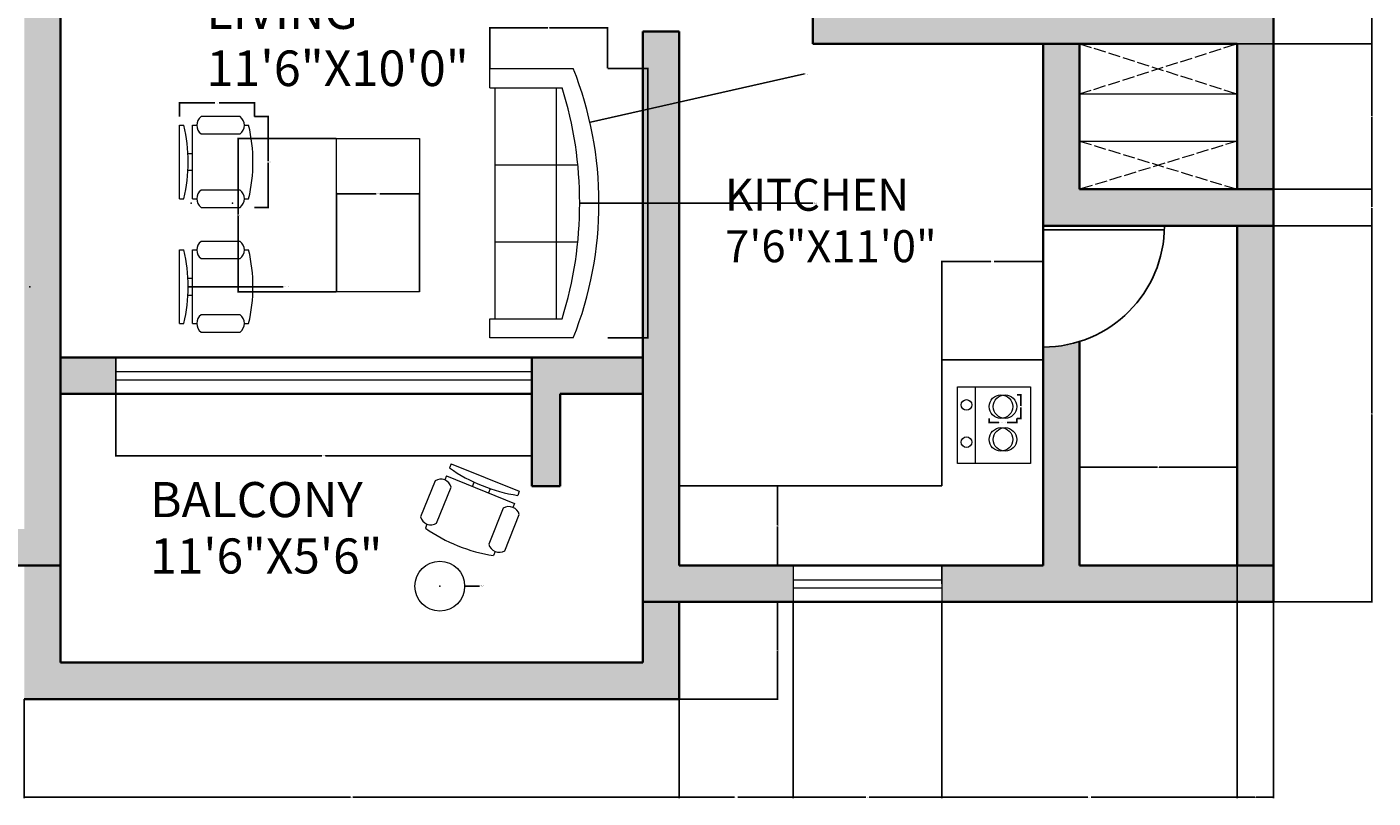
# Model space of a CAD drawing. Units: inches. Extents: x 582 to 1090, y 270 to 781.
# Tile 2 of 5: x 757 to 1090, y 270 to 461. Entities that reach past the tile are written whole.
import ezdxf

# ---------------------------------------------------------------- set-up
doc = ezdxf.new("R2010")
doc.units = ezdxf.units.IN
doc.header["$MEASUREMENT"] = 0
doc.linetypes.add('ACAD_ISO02W100', pattern=[15, 12, -3])
for name, color, linetype, lineweight in [('A-ANNO-DIMS', 2, 'Continuous', 18), ('A-AREA-IDEN', 7, 'Continuous', 25), ('A-DOOR', 3, 'Continuous', 25), ('A-EQPM', 8, 'Continuous', 18), ('A-FLOR-CASE', 32, 'Continuous', 25), ('A-FLOR-OPEN', 7, 'Continuous', 18), ('A-FLOR-OPEN-IDEN', 8, 'ACAD_ISO02W100', 13), ('A-FURN', 8, 'Continuous', 18), ('A-GLAZ', 4, 'Continuous', 18), ('A-WALL', 7, 'Continuous', 35)]:
    doc.layers.add(name, color=color, linetype=linetype, lineweight=lineweight)
doc.layers.add('A-WALL-PATT', color=9, linetype='Continuous', lineweight=13, true_color=0xc7c8ca)
doc.styles.get("Standard").update_dxf_attribs({"font": 'arial.ttf'})
doc.dimstyles.get("Standard").update_dxf_attribs({"dimtxt": 0.18, "dimasz": 0.18, "dimexe": 0.18, "dimexo": 0.0625, "dimgap": 0.09, "dimtad": 0, "dimtih": 1, "dimtoh": 1, "dimdec": 0, "dimzin": 0, "dimdsep": 46, "dimlunit": 3, "dimtxsty": 'Standard', "dimcen": 0.09, "dimadec": 0, "dimazin": 0, "dimtfac": 1, "dimtdec": 0, "dimtofl": 0, "dimtmove": 0, "dimatfit": 3, "dimfxl": 1, "dimtolj": 1, "dimtzin": 0, "dimarcsym": 0})

# ---------------------------------------------------------------- blocks, each defined once
blk = doc.blocks.new('Sofa - Roundback 7 ft.')
for p, q in [((-12.00002, -32.4421), (-12.00003, -6.5971)), ((11.99997, -32.4421), (11.99998, -6.5971)), ((-36.000027, -34), (-36.000027, -11.4696)), ((35.99998, -34), (35.99998, -11.4696)), ((-35.999844, -13.3819), (35.9998, -13.3819)), ((-36.000027, -32.4421), (35.99998, -32.4421))]:
    blk.add_line(p, q)
for points in [[(-36.000027, -34), (-42.000027, -34), (-42.000027, -8)], [(41.99998, -8), (41.99998, -34), (35.99998, -34)]]:
    blk.add_lwpolyline(points)
for centre, radius, start, end in [((0, -114.25), 114.25, 68.43141, 111.5686), ((-0.00001, -127.1968), 121.1968, 72.72033, 107.2797)]:
    blk.add_arc(centre, radius, start, end)
blk = doc.blocks.new('Chair - Desk')
for p, q in [((-8.5, 0), (-8.5, -1)), ((-8.5, 0), (8.5, 0)), ((8.5, 0), (8.5, -1)), ((-8.5, -3), (-8.5, -4)), ((-8.5, -3), (8.5, -3)), ((-2, -3), (-2, -1.9355)), ((2, -1.9576), (2, -3)), ((8.5, -3), (8.5, -4)), ((-10.5, -5), (-10.5, -14)), ((-6.5, -14), (-6.5, -5)), ((6.5, -5), (6.5, -14)), ((10.5, -14), (10.5, -5)), ((-8.5, -15), (-8.5, -16)), ((8.5, -15), (8.5, -16))]:
    blk.add_line(p, q)
for centre, radius, start, end in [((0, 34.625), 36.625, 256.5803, 283.4197), ((-8.5, -6.5), 2.5, 36.8699, 143.1301), ((8.5, -6.5), 2.5, 36.8699, 143.1301), ((-8.5, -12.5), 2.5, 216.8699, 323.1301), ((8.5, -12.5), 2.5, 216.8699, 323.1301), ((0, 19.625), 36.625, 256.5803, 283.4197)]:
    blk.add_arc(centre, radius, start, end)
blk = doc.blocks.new('DOOR-SINGLE-30IN')
for p, q in [((29, 0), (29, 30)), ((30, 0), (30, 30))]:
    blk.add_line(p, q)
blk.add_arc((30, 0), 30, 90, 180)
blk = doc.blocks.new('COOKTOP-BURNER')
for centre in [(2.91, 2.91), (3.92, 2.91)]:
    blk.add_circle(centre, 2.91)
blk = doc.blocks.new('*D22')
at = {"layer": 'A-ANNO-DIMS', "color": 0, "lineweight": -2, "transparency": 16777216}
for p, q in [((901.12, 450.33), (911.24, 450.33)), ((911.06, 450.15), (911.06, 417.2)), ((911.06, 383.89), (911.06, 416.84)), ((901.12, 383.71), (911.24, 383.71))]:
    blk.add_line(p, q, dxfattribs=at)
at = {"layer": 'A-ANNO-DIMS', "color": 0, "transparency": 16777216}
for points in [[(911.03, 450.15), (911.09, 450.15), (911.06, 450.33)], [(911.03, 383.89), (911.09, 383.89), (911.06, 383.71)]]:
    blk.add_solid(points, dxfattribs=at)
at = {"layer": 'Defpoints', "color": 0, "transparency": 16777216}
for p in [(901.06, 450.33), (901.06, 383.71), (911.06, 383.71)]:
    blk.add_point(p, dxfattribs=at)
at = {"layer": 'A-ANNO-DIMS', "color": 0, "transparency": 16777216, "insert": (911.06, 417.02), "char_height": 0.18, "attachment_point": 5}
blk.add_mtext('\\A1;SOFA 67', dxfattribs=at)
blk = doc.blocks.new('*D23')
at = {"layer": 'A-ANNO-DIMS', "color": 0, "lineweight": -2, "transparency": 16777216}
for p, q in [((871.98, 450.39), (871.98, 460.51)), ((872.16, 460.33), (886.3, 460.33)), ((900.88, 460.33), (886.74, 460.33)), ((901.06, 450.39), (901.06, 460.51))]:
    blk.add_line(p, q, dxfattribs=at)
at = {"layer": 'A-ANNO-DIMS', "color": 0, "transparency": 16777216}
for points in [[(872.16, 460.36), (872.16, 460.3), (871.98, 460.33)], [(900.88, 460.36), (900.88, 460.3), (901.06, 460.33)]]:
    blk.add_solid(points, dxfattribs=at)
at = {"layer": 'Defpoints', "color": 0, "transparency": 16777216}
for p in [(901.06, 460.33), (871.98, 450.33), (901.06, 450.33)]:
    blk.add_point(p, dxfattribs=at)
at = {"layer": 'A-ANNO-DIMS', "color": 0, "transparency": 16777216, "insert": (886.52, 460.33), "char_height": 0.18, "attachment_point": 5}
blk.add_mtext('\\A1;29', dxfattribs=at)
blk = doc.blocks.new('*D24')
at = {"layer": 'A-ANNO-DIMS', "color": 0, "lineweight": -2, "transparency": 16777216}
for p, q in [((813.79, 438.43), (817.28, 438.43)), ((817.1, 438.25), (817.1, 427.39)), ((817.1, 416.17), (817.1, 427.02)), ((813.79, 415.99), (817.28, 415.99))]:
    blk.add_line(p, q, dxfattribs=at)
at = {"layer": 'A-ANNO-DIMS', "color": 0, "transparency": 16777216}
for points in [[(817.07, 438.25), (817.13, 438.25), (817.1, 438.43)], [(817.07, 416.17), (817.13, 416.17), (817.1, 415.99)]]:
    blk.add_solid(points, dxfattribs=at)
at = {"layer": 'Defpoints', "color": 0, "transparency": 16777216}
for p in [(813.73, 438.43), (817.1, 438.43), (813.73, 415.99)]:
    blk.add_point(p, dxfattribs=at)
at = {"layer": 'A-ANNO-DIMS', "color": 0, "transparency": 16777216, "insert": (817.1, 427.21), "char_height": 0.18, "attachment_point": 5}
blk.add_mtext('\\A1;CHAIR 22 TYP.', dxfattribs=at)
blk = doc.blocks.new('*D25')
at = {"layer": 'A-ANNO-DIMS', "color": 0, "lineweight": -2, "transparency": 16777216}
for p, q in [((795.21, 438.49), (795.21, 441.97)), ((795.39, 441.79), (803.95, 441.79)), ((813.55, 441.79), (804.99, 441.79)), ((813.73, 438.49), (813.73, 441.97))]:
    blk.add_line(p, q, dxfattribs=at)
at = {"layer": 'A-ANNO-DIMS', "color": 0, "transparency": 16777216}
for points in [[(795.39, 441.82), (795.39, 441.76), (795.21, 441.79)], [(813.55, 441.82), (813.55, 441.76), (813.73, 441.79)]]:
    blk.add_solid(points, dxfattribs=at)
at = {"layer": 'Defpoints', "color": 0, "transparency": 16777216}
for p in [(795.21, 441.79), (795.21, 438.43), (813.73, 438.43)]:
    blk.add_point(p, dxfattribs=at)
at = {"layer": 'A-ANNO-DIMS', "color": 0, "transparency": 16777216, "insert": (804.47, 441.79), "char_height": 0.18, "attachment_point": 5}
blk.add_mtext('\\A1;19 TYP.', dxfattribs=at)
blk = doc.blocks.new('*D32')
at = {"layer": 'A-ANNO-DIMS', "color": 0, "lineweight": -2, "transparency": 16777216}
for p, q in [((995.45, 363.75), (995.45, 362.61)), ((1002.28, 363.75), (1002.28, 362.61)), ((995.63, 362.79), (997.85, 362.79)), ((1002.1, 362.79), (999.89, 362.79))]:
    blk.add_line(p, q, dxfattribs=at)
at = {"layer": 'A-ANNO-DIMS', "color": 0, "transparency": 16777216}
for points in [[(995.63, 362.82), (995.63, 362.76), (995.45, 362.79)], [(1002.1, 362.82), (1002.1, 362.76), (1002.28, 362.79)]]:
    blk.add_solid(points, dxfattribs=at)
at = {"layer": 'Defpoints', "color": 0, "transparency": 16777216}
for p in [(995.45, 363.81), (1002.28, 363.81), (1002.28, 362.79)]:
    blk.add_point(p, dxfattribs=at)
at = {"layer": 'A-ANNO-DIMS', "color": 0, "transparency": 16777216, "insert": (998.87, 362.79), "char_height": 0.18, "attachment_point": 5}
blk.add_mtext('\\A1;BURNER 7 TYP.', dxfattribs=at)
blk = doc.blocks.new('*D33')
at = {"layer": 'A-ANNO-DIMS', "color": 0, "lineweight": -2, "transparency": 16777216}
for p, q in [((1002.35, 369.64), (1003.49, 369.64)), ((1003.31, 369.46), (1003.31, 366.91)), ((1003.31, 363.99), (1003.31, 366.54)), ((1002.35, 363.81), (1003.49, 363.81))]:
    blk.add_line(p, q, dxfattribs=at)
at = {"layer": 'A-ANNO-DIMS', "color": 0, "transparency": 16777216}
for points in [[(1003.28, 369.46), (1003.34, 369.46), (1003.31, 369.64)], [(1003.28, 363.99), (1003.34, 363.99), (1003.31, 363.81)]]:
    blk.add_solid(points, dxfattribs=at)
at = {"layer": 'Defpoints', "color": 0, "transparency": 16777216}
for p in [(1002.28, 369.64), (1003.31, 369.64), (1002.28, 363.81)]:
    blk.add_point(p, dxfattribs=at)
at = {"layer": 'A-ANNO-DIMS', "color": 0, "transparency": 16777216, "insert": (1003.31, 366.72), "char_height": 0.18, "attachment_point": 5}
blk.add_mtext('\\A1;6 TYP.', dxfattribs=at)
blk = doc.blocks.new('*D38')
at = {"layer": 'A-ANNO-DIMS', "color": 0, "lineweight": -2, "transparency": 16777216}
for p, q in [((918.87, 318.45), (943.28, 318.45)), ((943.1, 318.27), (943.1, 306.62)), ((943.1, 294.62), (943.1, 306.26)), ((918.87, 294.44), (943.28, 294.44))]:
    blk.add_line(p, q, dxfattribs=at)
at = {"layer": 'A-ANNO-DIMS', "color": 0, "transparency": 16777216}
for points in [[(943.07, 318.27), (943.13, 318.27), (943.1, 318.45)], [(943.07, 294.62), (943.13, 294.62), (943.1, 294.44)]]:
    blk.add_solid(points, dxfattribs=at)
at = {"layer": 'Defpoints', "color": 0, "transparency": 16777216}
for p in [(918.8, 318.45), (918.8, 294.44), (943.1, 294.44)]:
    blk.add_point(p, dxfattribs=at)
at = {"layer": 'A-ANNO-DIMS', "color": 0, "transparency": 16777216, "insert": (943.1, 306.44), "char_height": 0.18, "attachment_point": 5}
blk.add_mtext('\\A1;24.01', dxfattribs=at)
blk = doc.blocks.new('*D39')
at = {"layer": 'A-ANNO-DIMS', "color": 0, "lineweight": -2, "transparency": 16777216}
for p, q in [((756.8, 294.37), (756.8, 269.96)), ((918.8, 294.37), (918.8, 269.96)), ((756.98, 270.14), (837.53, 270.14)), ((918.62, 270.14), (838.08, 270.14))]:
    blk.add_line(p, q, dxfattribs=at)
at = {"layer": 'A-ANNO-DIMS', "color": 0, "transparency": 16777216}
for points in [[(756.98, 270.17), (756.98, 270.11), (756.8, 270.14)], [(918.62, 270.17), (918.62, 270.11), (918.8, 270.14)]]:
    blk.add_solid(points, dxfattribs=at)
at = {"layer": 'Defpoints', "color": 0, "transparency": 16777216}
for p in [(756.8, 294.44), (918.8, 294.44), (918.8, 270.14)]:
    blk.add_point(p, dxfattribs=at)
at = {"layer": 'A-ANNO-DIMS', "color": 0, "transparency": 16777216, "insert": (837.8, 270.14), "char_height": 0.18, "attachment_point": 5}
blk.add_mtext('\\A1;162', dxfattribs=at)
blk = doc.blocks.new('*D43')
at = {"layer": 'A-ANNO-DIMS', "color": 0, "lineweight": -2, "transparency": 16777216}
for p, q in [((918.8, 318.38), (918.8, 269.96)), ((946.96, 318.38), (946.96, 269.96)), ((918.98, 270.14), (932.49, 270.14)), ((946.78, 270.14), (933.28, 270.14))]:
    blk.add_line(p, q, dxfattribs=at)
at = {"layer": 'A-ANNO-DIMS', "color": 0, "transparency": 16777216}
for points in [[(918.98, 270.17), (918.98, 270.11), (918.8, 270.14)], [(946.78, 270.17), (946.78, 270.11), (946.96, 270.14)]]:
    blk.add_solid(points, dxfattribs=at)
at = {"layer": 'Defpoints', "color": 0, "transparency": 16777216}
for p in [(918.8, 318.45), (946.96, 318.45), (946.96, 270.14)]:
    blk.add_point(p, dxfattribs=at)
at = {"layer": 'A-ANNO-DIMS', "color": 0, "transparency": 16777216, "insert": (932.88, 270.14), "char_height": 0.18, "attachment_point": 5}
blk.add_mtext('\\A1;28.16', dxfattribs=at)
blk = doc.blocks.new('*D44')
at = {"layer": 'A-ANNO-DIMS', "color": 0, "lineweight": -2, "transparency": 16777216}
for p, q in [((946.96, 318.38), (946.96, 269.96)), ((983.73, 318.38), (983.73, 269.96)), ((947.14, 270.14), (964.95, 270.14)), ((983.55, 270.14), (965.74, 270.14))]:
    blk.add_line(p, q, dxfattribs=at)
at = {"layer": 'A-ANNO-DIMS', "color": 0, "transparency": 16777216}
for points in [[(947.14, 270.17), (947.14, 270.11), (946.96, 270.14)], [(983.55, 270.17), (983.55, 270.11), (983.73, 270.14)]]:
    blk.add_solid(points, dxfattribs=at)
at = {"layer": 'Defpoints', "color": 0, "transparency": 16777216}
for p in [(946.96, 318.45), (983.73, 318.45), (983.73, 270.14)]:
    blk.add_point(p, dxfattribs=at)
at = {"layer": 'A-ANNO-DIMS', "color": 0, "transparency": 16777216, "insert": (965.35, 270.14), "char_height": 0.18, "attachment_point": 5}
blk.add_mtext('\\A1;36.77', dxfattribs=at)
blk = doc.blocks.new('*D45')
at = {"layer": 'A-ANNO-DIMS', "color": 0, "lineweight": -2, "transparency": 16777216}
for p, q in [((1056.8, 327.38), (1056.8, 269.96)), ((983.73, 318.38), (983.73, 269.96)), ((983.91, 270.14), (1019.88, 270.14)), ((1056.62, 270.14), (1020.66, 270.14))]:
    blk.add_line(p, q, dxfattribs=at)
at = {"layer": 'A-ANNO-DIMS', "color": 0, "transparency": 16777216}
for points in [[(983.91, 270.17), (983.91, 270.11), (983.73, 270.14)], [(1056.62, 270.17), (1056.62, 270.11), (1056.8, 270.14)]]:
    blk.add_solid(points, dxfattribs=at)
at = {"layer": 'Defpoints', "color": 0, "transparency": 16777216}
for p in [(1056.8, 327.45), (983.73, 318.45), (1056.8, 270.14)]:
    blk.add_point(p, dxfattribs=at)
at = {"layer": 'A-ANNO-DIMS', "color": 0, "transparency": 16777216, "insert": (1020.27, 270.14), "char_height": 0.18, "attachment_point": 5}
blk.add_mtext('\\A1;73.07', dxfattribs=at)
blk = doc.blocks.new('*D46')
at = {"layer": 'A-ANNO-DIMS', "color": 0, "lineweight": -2, "transparency": 16777216}
for p, q in [((1056.8, 327.38), (1056.8, 269.96)), ((1065.8, 318.38), (1065.8, 269.96)), ((1056.98, 270.14), (1061.16, 270.14)), ((1065.62, 270.14), (1061.45, 270.14))]:
    blk.add_line(p, q, dxfattribs=at)
at = {"layer": 'A-ANNO-DIMS', "color": 0, "transparency": 16777216}
for points in [[(1056.98, 270.17), (1056.98, 270.11), (1056.8, 270.14)], [(1065.62, 270.17), (1065.62, 270.11), (1065.8, 270.14)]]:
    blk.add_solid(points, dxfattribs=at)
at = {"layer": 'Defpoints', "color": 0, "transparency": 16777216}
for p in [(1056.8, 327.45), (1065.8, 318.45), (1065.8, 270.14)]:
    blk.add_point(p, dxfattribs=at)
at = {"layer": 'A-ANNO-DIMS', "color": 0, "transparency": 16777216, "insert": (1061.3, 270.14), "char_height": 0.18, "attachment_point": 5}
blk.add_mtext('\\A1;9', dxfattribs=at)
blk = doc.blocks.new('*D47')
at = {"layer": 'A-ANNO-DIMS', "color": 0, "lineweight": -2, "transparency": 16777216}
for p, q in [((779.42, 378.81), (779.42, 354.39)), ((882.35, 378.81), (882.35, 354.39)), ((779.6, 354.57), (830.43, 354.57)), ((882.17, 354.57), (831.34, 354.57))]:
    blk.add_line(p, q, dxfattribs=at)
at = {"layer": 'A-ANNO-DIMS', "color": 0, "transparency": 16777216}
for points in [[(779.6, 354.6), (779.6, 354.54), (779.42, 354.57)], [(882.17, 354.6), (882.17, 354.54), (882.35, 354.57)]]:
    blk.add_solid(points, dxfattribs=at)
at = {"layer": 'Defpoints', "color": 0, "transparency": 16777216}
for p in [(779.42, 378.87), (882.35, 378.87), (779.42, 354.57)]:
    blk.add_point(p, dxfattribs=at)
at = {"layer": 'A-ANNO-DIMS', "color": 0, "transparency": 16777216, "insert": (830.89, 354.57), "char_height": 0.18, "attachment_point": 5}
blk.add_mtext('\\A1;102.93', dxfattribs=at)
blk = doc.blocks.new('*D58')
at = {"layer": 'A-ANNO-DIMS', "color": 0, "lineweight": -2, "transparency": 16777216}
for p, q in [((1065.87, 478.21), (1090.28, 478.21)), ((1090.1, 478.03), (1090.1, 467.51)), ((1090.1, 456.63), (1090.1, 467.15)), ((1056.87, 456.45), (1090.28, 456.45))]:
    blk.add_line(p, q, dxfattribs=at)
at = {"layer": 'A-ANNO-DIMS', "color": 0, "transparency": 16777216}
for points in [[(1090.07, 478.03), (1090.13, 478.03), (1090.1, 478.21)], [(1090.07, 456.63), (1090.13, 456.63), (1090.1, 456.45)]]:
    blk.add_solid(points, dxfattribs=at)
at = {"layer": 'Defpoints', "color": 0, "transparency": 16777216}
for p in [(1065.8, 478.21), (1090.1, 478.21), (1056.8, 456.45)]:
    blk.add_point(p, dxfattribs=at)
at = {"layer": 'A-ANNO-DIMS', "color": 0, "transparency": 16777216, "insert": (1090.1, 467.33), "char_height": 0.18, "attachment_point": 5}
blk.add_mtext('\\A1;21.77', dxfattribs=at)
blk = doc.blocks.new('*D59')
at = {"layer": 'A-ANNO-DIMS', "color": 0, "lineweight": -2, "transparency": 16777216}
for p, q in [((1056.87, 456.45), (1090.28, 456.45)), ((1090.1, 456.27), (1090.1, 438.63)), ((1090.1, 420.63), (1090.1, 438.26)), ((1056.87, 420.45), (1090.28, 420.45))]:
    blk.add_line(p, q, dxfattribs=at)
at = {"layer": 'A-ANNO-DIMS', "color": 0, "transparency": 16777216}
for points in [[(1090.07, 456.27), (1090.13, 456.27), (1090.1, 456.45)], [(1090.07, 420.63), (1090.13, 420.63), (1090.1, 420.45)]]:
    blk.add_solid(points, dxfattribs=at)
at = {"layer": 'Defpoints', "color": 0, "transparency": 16777216}
for p in [(1056.8, 456.45), (1090.1, 456.45), (1056.8, 420.45)]:
    blk.add_point(p, dxfattribs=at)
at = {"layer": 'A-ANNO-DIMS', "color": 0, "transparency": 16777216, "insert": (1090.1, 438.45), "char_height": 0.18, "attachment_point": 5}
blk.add_mtext('\\A1;36', dxfattribs=at)
blk = doc.blocks.new('*D60')
at = {"layer": 'A-ANNO-DIMS', "color": 0, "lineweight": -2, "transparency": 16777216}
for p, q in [((1056.87, 420.45), (1090.28, 420.45)), ((1090.1, 420.27), (1090.1, 416.13)), ((1090.1, 411.63), (1090.1, 415.76)), ((1065.87, 411.45), (1090.28, 411.45))]:
    blk.add_line(p, q, dxfattribs=at)
at = {"layer": 'A-ANNO-DIMS', "color": 0, "transparency": 16777216}
for points in [[(1090.07, 420.27), (1090.13, 420.27), (1090.1, 420.45)], [(1090.07, 411.63), (1090.13, 411.63), (1090.1, 411.45)]]:
    blk.add_solid(points, dxfattribs=at)
at = {"layer": 'Defpoints', "color": 0, "transparency": 16777216}
for p in [(1056.8, 420.45), (1090.1, 420.45), (1065.8, 411.45)]:
    blk.add_point(p, dxfattribs=at)
at = {"layer": 'A-ANNO-DIMS', "color": 0, "transparency": 16777216, "insert": (1090.1, 415.95), "char_height": 0.18, "attachment_point": 5}
blk.add_mtext('\\A1;9', dxfattribs=at)
blk = doc.blocks.new('*D61')
at = {"layer": 'A-ANNO-DIMS', "color": 0, "lineweight": -2, "transparency": 16777216}
for p, q in [((1065.87, 411.45), (1090.28, 411.45)), ((1090.1, 411.27), (1090.1, 365.13)), ((1090.1, 318.63), (1090.1, 364.76)), ((1065.87, 318.45), (1090.28, 318.45))]:
    blk.add_line(p, q, dxfattribs=at)
at = {"layer": 'A-ANNO-DIMS', "color": 0, "transparency": 16777216}
for points in [[(1090.07, 411.27), (1090.13, 411.27), (1090.1, 411.45)], [(1090.07, 318.63), (1090.13, 318.63), (1090.1, 318.45)]]:
    blk.add_solid(points, dxfattribs=at)
at = {"layer": 'Defpoints', "color": 0, "transparency": 16777216}
for p in [(1065.8, 411.45), (1090.1, 411.45), (1065.8, 318.45)]:
    blk.add_point(p, dxfattribs=at)
at = {"layer": 'A-ANNO-DIMS', "color": 0, "transparency": 16777216, "insert": (1090.1, 364.95), "char_height": 0.18, "attachment_point": 5}
blk.add_mtext('\\A1;93', dxfattribs=at)
blk = doc.blocks.new('*D62')
at = {"layer": 'A-ANNO-DIMS', "color": 0, "lineweight": -2, "transparency": 16777216}
for p, q in [((1017.8, 327.51), (1017.8, 351.93)), ((1017.98, 351.75), (1037.09, 351.75)), ((1056.62, 351.75), (1037.52, 351.75)), ((1056.8, 327.51), (1056.8, 351.93))]:
    blk.add_line(p, q, dxfattribs=at)
at = {"layer": 'A-ANNO-DIMS', "color": 0, "transparency": 16777216}
for points in [[(1017.98, 351.78), (1017.98, 351.72), (1017.8, 351.75)], [(1056.62, 351.78), (1056.62, 351.72), (1056.8, 351.75)]]:
    blk.add_solid(points, dxfattribs=at)
at = {"layer": 'Defpoints', "color": 0, "transparency": 16777216}
for p in [(1056.8, 351.75), (1017.8, 327.45), (1056.8, 327.45)]:
    blk.add_point(p, dxfattribs=at)
at = {"layer": 'A-ANNO-DIMS', "color": 0, "transparency": 16777216, "insert": (1037.3, 351.75), "char_height": 0.18, "attachment_point": 5}
blk.add_mtext('\\A1;39', dxfattribs=at)
blk = doc.blocks.new('*D63')
at = {"layer": 'A-ANNO-DIMS', "color": 0, "lineweight": -2, "transparency": 16777216}
for p, q in [((834.01, 395.13), (834.01, 419.55)), ((854.57, 395.13), (854.57, 419.55)), ((834.19, 419.37), (843.82, 419.37)), ((854.39, 419.37), (844.75, 419.37))]:
    blk.add_line(p, q, dxfattribs=at)
at = {"layer": 'A-ANNO-DIMS', "color": 0, "transparency": 16777216}
for points in [[(834.19, 419.4), (834.19, 419.34), (834.01, 419.37)], [(854.39, 419.4), (854.39, 419.34), (854.57, 419.37)]]:
    blk.add_solid(points, dxfattribs=at)
at = {"layer": 'Defpoints', "color": 0, "transparency": 16777216}
for p in [(854.57, 419.37), (834.01, 395.07), (854.57, 395.07)]:
    blk.add_point(p, dxfattribs=at)
at = {"layer": 'A-ANNO-DIMS', "color": 0, "transparency": 16777216, "insert": (844.29, 419.37), "char_height": 0.18, "attachment_point": 5}
blk.add_mtext('\\A1;20.563', dxfattribs=at)
blk = doc.blocks.new('*D64')
at = {"layer": 'A-ANNO-DIMS', "color": 0, "lineweight": -2, "transparency": 16777216}
for p, q in [((833.94, 433.04), (809.53, 433.04)), ((809.71, 432.86), (809.71, 414.24)), ((809.71, 395.25), (809.71, 413.87)), ((833.94, 395.07), (809.53, 395.07))]:
    blk.add_line(p, q, dxfattribs=at)
at = {"layer": 'A-ANNO-DIMS', "color": 0, "transparency": 16777216}
for points in [[(809.68, 432.86), (809.74, 432.86), (809.71, 433.04)], [(809.68, 395.25), (809.74, 395.25), (809.71, 395.07)]]:
    blk.add_solid(points, dxfattribs=at)
at = {"layer": 'Defpoints', "color": 0, "transparency": 16777216}
for p in [(809.71, 433.04), (834.01, 433.04), (834.01, 395.07)]:
    blk.add_point(p, dxfattribs=at)
at = {"layer": 'A-ANNO-DIMS', "color": 0, "transparency": 16777216, "insert": (809.71, 414.05), "char_height": 0.18, "attachment_point": 5}
blk.add_mtext('\\A1;37.98', dxfattribs=at)
blk = doc.blocks.new('*D65')
at = {"layer": 'A-ANNO-DIMS', "color": 0, "lineweight": -2, "transparency": 16777216}
for p, q in [((983.77, 378.34), (983.77, 402.76)), ((983.95, 402.58), (995.89, 402.58)), ((1008.62, 402.58), (996.68, 402.58)), ((1008.8, 378.34), (1008.8, 402.76))]:
    blk.add_line(p, q, dxfattribs=at)
at = {"layer": 'A-ANNO-DIMS', "color": 0, "transparency": 16777216}
for points in [[(983.95, 402.61), (983.95, 402.55), (983.77, 402.58)], [(1008.62, 402.61), (1008.62, 402.55), (1008.8, 402.58)]]:
    blk.add_solid(points, dxfattribs=at)
at = {"layer": 'Defpoints', "color": 0, "transparency": 16777216}
for p in [(1008.8, 402.58), (983.77, 378.28), (1008.8, 378.28)]:
    blk.add_point(p, dxfattribs=at)
at = {"layer": 'A-ANNO-DIMS', "color": 0, "transparency": 16777216, "insert": (996.29, 402.58), "char_height": 0.18, "attachment_point": 5}
blk.add_mtext('\\A1;25.03', dxfattribs=at)
blk = doc.blocks.new('*D66')
at = {"layer": 'A-ANNO-DIMS', "color": 0, "lineweight": -2, "transparency": 16777216}
for p, q in [((918.87, 347.11), (943.28, 347.11)), ((943.1, 346.93), (943.1, 337.46)), ((943.1, 327.63), (943.1, 337.1)), ((918.87, 327.45), (943.28, 327.45))]:
    blk.add_line(p, q, dxfattribs=at)
at = {"layer": 'A-ANNO-DIMS', "color": 0, "transparency": 16777216}
for points in [[(943.07, 346.93), (943.13, 346.93), (943.1, 347.11)], [(943.07, 327.63), (943.13, 327.63), (943.1, 327.45)]]:
    blk.add_solid(points, dxfattribs=at)
at = {"layer": 'Defpoints', "color": 0, "transparency": 16777216}
for p in [(918.8, 347.11), (918.8, 327.45), (943.1, 327.45)]:
    blk.add_point(p, dxfattribs=at)
at = {"layer": 'A-ANNO-DIMS', "color": 0, "transparency": 16777216, "insert": (943.1, 337.28), "char_height": 0.18, "attachment_point": 5}
blk.add_mtext('\\A1;19.668', dxfattribs=at)
blk = doc.blocks.new('*D67')
at = {"layer": 'A-ANNO-DIMS', "color": 0, "lineweight": -2, "transparency": 16777216}
for p, q in [((859.48, 322.35), (859.66, 322.35)), ((859.57, 322.26), (859.57, 322.44)), ((869.43, 322.35), (865.91, 322.35))]:
    blk.add_line(p, q, dxfattribs=at)
at = {"layer": 'A-ANNO-DIMS', "color": 0, "transparency": 16777216}
blk.add_solid([(865.91, 322.38), (865.91, 322.32), (865.73, 322.35)], dxfattribs=at)
at = {"layer": 'Defpoints', "color": 0, "transparency": 16777216}
for p in [(853.41, 322.34), (865.73, 322.35)]:
    blk.add_point(p, dxfattribs=at)
at = {"layer": 'A-ANNO-DIMS', "color": 0, "transparency": 16777216, "insert": (869.99, 322.35), "char_height": 0.18, "attachment_point": 5}
blk.add_mtext('\\A1;∅12.317', dxfattribs=at)
blk = doc.blocks.new('*D70')
at = {"layer": 'A-ANNO-DIMS', "color": 0, "lineweight": -2, "transparency": 16777216}
for p, q in [((797.97, 417.02), (798.15, 417.02)), ((798.06, 416.93), (798.06, 417.11)), ((951.86, 417.02), (894.37, 417.02))]:
    blk.add_line(p, q, dxfattribs=at)
at = {"layer": 'A-ANNO-DIMS', "color": 0, "transparency": 16777216}
blk.add_solid([(894.37, 417.05), (894.37, 416.99), (894.19, 417.02)], dxfattribs=at)
at = {"layer": 'Defpoints', "color": 0, "transparency": 16777216}
for p in [(798.06, 417.02), (894.19, 417.02)]:
    blk.add_point(p, dxfattribs=at)
at = {"layer": 'A-ANNO-DIMS', "color": 0, "transparency": 16777216, "insert": (952.34, 417.02), "char_height": 0.18, "attachment_point": 5}
blk.add_mtext('\\A1;R96.13', dxfattribs=at)
blk = doc.blocks.new('*D73')
at = {"layer": 'A-ANNO-DIMS', "color": 0, "lineweight": -2, "transparency": 16777216}
for p, q in [((949.75, 448.98), (896.89, 437.03)), ((808.24, 417.02), (808.42, 417.02)), ((808.33, 416.93), (808.33, 417.11))]:
    blk.add_line(p, q, dxfattribs=at)
at = {"layer": 'A-ANNO-DIMS', "color": 0, "transparency": 16777216}
blk.add_solid([(896.89, 437.06), (896.9, 437), (896.72, 436.99)], dxfattribs=at)
at = {"layer": 'Defpoints', "color": 0, "transparency": 16777216}
for p in [(896.72, 436.99), (808.33, 417.02)]:
    blk.add_point(p, dxfattribs=at)
at = {"layer": 'A-ANNO-DIMS', "color": 0, "transparency": 16777216, "insert": (950.23, 448.98), "char_height": 0.18, "attachment_point": 5}
blk.add_mtext('\\A1;R90.62', dxfattribs=at)
blk = doc.blocks.new('*D77')
at = {"layer": 'A-ANNO-DIMS', "color": 0, "lineweight": -2, "transparency": 16777216}
for p, q in [((758.12, 396.37), (758.3, 396.37)), ((758.21, 396.28), (758.21, 396.46)), ((820.83, 396.37), (797.53, 396.37))]:
    blk.add_line(p, q, dxfattribs=at)
at = {"layer": 'A-ANNO-DIMS', "color": 0, "transparency": 16777216}
blk.add_solid([(797.53, 396.4), (797.53, 396.34), (797.35, 396.37)], dxfattribs=at)
at = {"layer": 'Defpoints', "color": 0, "transparency": 16777216}
for p in [(758.21, 396.37), (797.35, 396.37)]:
    blk.add_point(p, dxfattribs=at)
at = {"layer": 'A-ANNO-DIMS', "color": 0, "transparency": 16777216, "insert": (821.57, 396.37), "char_height": 0.18, "attachment_point": 5}
blk.add_mtext('\\A1;6X R39.136', dxfattribs=at)

msp = doc.modelspace()

# ---------------------------------------------------------------- hatches: boundary and pattern name
at = {"layer": 'A-WALL-PATT'}
h = msp.add_hatch(color=256, dxfattribs=at)
h.dxf.hatch_style = 1
h.paths.add_polyline_path([(867.8047, 744.446), (765.8047, 744.446), (606.8047, 744.446), (606.8047, 711.9379), (615.8047, 711.9379), (615.8047, 735.446), (756.8047, 735.446), (756.8047, 585.446), (765.8047, 585.446), (765.8047, 735.446), (868.9478, 735.446, -0.06325422)])
h.paths.add_polyline_path([(1065.8047, 744.446), (912.8047, 744.446), (903.8047, 744.446), (903.8047, 708.446), (903.8047, 594.446), (903.8047, 564.6071), (912.8047, 564.6071), (912.8047, 600.6071), (912.8047, 735.446), (1056.8047, 735.446), (1056.8047, 720.2375), (1065.8047, 720.2375)])
h.paths.add_polyline_path([(1065.8047, 632.4383), (1056.8047, 632.4383), (1056.8047, 594.446), (1056.8047, 584.9343), (1065.8047, 584.9343), (1065.8047, 594.446)], flags=17)
h.paths.add_polyline_path([(1056.8047, 603.446), (951.8047, 603.446), (951.8047, 594.446), (1056.8047, 594.446)], flags=17)
h.paths.add_polyline_path([(1065.8047, 525.446), (1065.8047, 550.2593), (1056.8047, 550.2593), (1056.8047, 534.446), (960.8047, 534.446), (960.8047, 565.946, -0.07397332), (952.1262, 564.6071), (951.8047, 564.6071), (951.8047, 495.446, -0.07632083), (960.8047, 494.0641), (960.8047, 525.446), (1056.8047, 525.446), (1056.8047, 508.8565), (1065.8047, 508.8565)])
h.paths.add_polyline_path([(1065.8047, 478.2143), (1056.8047, 478.2143), (1056.8047, 465.446), (951.8047, 465.446), (951.8047, 456.446), (1056.8047, 456.446), (1056.8047, 420.446), (1065.8047, 420.446), (1065.8047, 456.446)])
h.paths.add_polyline_path([(1065.8047, 420.446), (1056.8047, 420.446), (1017.8047, 420.446), (1017.8047, 456.446), (1008.8047, 456.446), (1008.8047, 411.446), (1038.8047, 411.446), (1065.8047, 411.446)])
h.paths.add_polyline_path([(1065.8047, 411.446), (1056.8047, 411.446), (1056.8047, 327.446), (1065.8047, 327.446)])
h.paths.add_polyline_path([(1065.8047, 327.446), (1056.8047, 327.446), (1017.8047, 327.446), (1017.8047, 382.8278, -0.07632083), (1008.8047, 381.446), (1008.8047, 327.446), (983.7348, 327.446), (983.7348, 318.446), (1065.8047, 318.446)])
h.paths.add_polyline_path([(946.9624, 327.446), (918.8047, 327.446), (918.8047, 369.8742), (918.8047, 459.446), (909.8047, 459.446), (909.8047, 369.8742), (909.8047, 318.446), (946.9624, 318.446)])
h.paths.add_polyline_path([(918.8047, 318.446), (909.8047, 318.446), (909.8047, 303.4372), (765.8047, 303.4372), (765.8047, 327.446), (756.8047, 327.446), (756.8047, 294.4372), (918.8047, 294.4372)])
h.paths.add_polyline_path([(909.8047, 378.8742), (882.3477, 378.8742), (882.3477, 347.0959), (889.3299, 347.0959), (889.3299, 369.8742), (909.8047, 369.8742)])
h.paths.add_polyline_path([(779.4225, 378.8742), (765.8047, 378.8742), (765.8047, 369.8742), (779.4225, 369.8742)])
h.paths.add_polyline_path([(765.8047, 516.446), (756.8047, 516.446), (756.8047, 480.446), (756.8047, 336.446), (724.1731, 336.446), (724.1731, 327.446), (765.8047, 327.446), (765.8047, 369.8742), (765.8047, 378.8742)])
h.paths.add_polyline_path([(615.8047, 516.446), (606.8047, 516.446), (606.8047, 327.446), (637.062, 327.446), (637.062, 336.446), (615.8047, 336.446)])
h.paths.add_polyline_path([(615.8047, 631.6498), (606.8047, 631.6498), (606.8047, 585.446), (606.8047, 569.338), (615.8047, 569.338), (615.8047, 585.446), (615.8047, 594.446)])
h.paths.add_polyline_path([(721.9478, 594.446), (615.8047, 594.446), (615.8047, 585.446), (627.9505, 585.446, -0.03261849), (629.8936, 585.446), (710.8047, 585.446), (710.8047, 525.446), (675.3033, 525.446), (675.3033, 516.446), (719.8047, 516.446), (720.8047, 516.446), (720.8047, 525.446), (719.8047, 525.446), (719.8047, 585.446), (720.8047, 585.446, -0.06325422)])
h.paths.add_polyline_path([(646.6852, 525.446), (615.8047, 525.446), (615.8047, 516.446), (645.3033, 516.446, -0.07632083)])
h.paths.add_polyline_path([(615.8047, 525.446), (615.8047, 539.7667), (606.8047, 539.7667), (606.8047, 516.446), (615.8047, 516.446)])

# ---------------------------------------------------------------- linework, layer by layer
at = {"layer": 'A-DOOR'}
msp.add_line((1008.8047, 411.446), (1008.8047, 381.446), dxfattribs=at)
at = {"layer": 'A-EQPM'}
msp.add_line((991.9866, 371.6418), (991.9866, 352.7025), dxfattribs=at)
msp.add_lwpolyline([(987.6109, 371.6418), (1005.6608, 371.6418), (1005.6608, 352.7025), (987.6109, 352.7025)], close=True, dxfattribs=at)
for centre in [(989.8491, 367.1465), (989.8491, 357.9529)]:
    msp.add_circle(centre, 1.3124, dxfattribs=at)
at = {"layer": 'A-FLOR-CASE'}
for p, q in [((1008.8047, 378.277), (983.7733, 378.277)), ((983.7733, 378.277), (983.7733, 347.1136)), ((983.7733, 347.1136), (918.8047, 347.1136))]:
    msp.add_line(p, q, dxfattribs=at)
at = {"layer": 'A-FLOR-OPEN'}
for p, q in [((1017.8047, 444.0264), (1056.8047, 444.0264)), ((1017.8047, 432.3711), (1056.8047, 432.3711))]:
    msp.add_line(p, q, dxfattribs=at)
at = {"layer": 'A-FLOR-OPEN-IDEN', "ltscale": 0.25}
for p, q in [((1017.8047, 456.446), (1056.8047, 444.0264)), ((1017.8047, 444.0264), (1056.8047, 456.446)), ((1017.8047, 432.3711), (1056.8047, 420.446)), ((1056.8047, 432.3711), (1017.8047, 420.446))]:
    msp.add_line(p, q, dxfattribs=at)
at = {"layer": 'A-FURN'}
msp.add_lwpolyline([(834.0061, 433.0436), (854.5691, 433.0436), (854.5691, 395.066), (834.0061, 395.066)], close=True, dxfattribs=at)
msp.add_circle((859.5721, 322.3463), 6.1583, dxfattribs=at)
at = {"layer": 'A-GLAZ'}
for p, q in [((779.4225, 369.8742), (779.4225, 378.8742)), ((779.4225, 375.3742), (882.3477, 375.3742)), ((779.4225, 373.3742), (882.3477, 373.3742)), ((946.9624, 327.446), (946.9624, 318.446)), ((983.7348, 322.946), (983.7348, 327.446)), ((983.7348, 327.446), (983.7348, 318.446)), ((946.9624, 323.946), (983.7348, 323.946)), ((946.9624, 321.946), (983.7348, 321.946))]:
    msp.add_line(p, q, dxfattribs=at)
at = {"layer": 'A-WALL'}
for p, q in [((1065.8047, 594.446), (1065.8047, 318.446)), ((765.8047, 327.446), (765.8047, 516.446)), ((765.8047, 516.446), (765.8047, 396.446)), ((951.8047, 456.446), (951.8047, 466.446)), ((918.8047, 459.446), (909.8047, 459.446)), ((909.8047, 459.446), (909.8047, 369.8742)), ((918.8047, 327.446), (918.8047, 459.446)), ((1056.8047, 456.446), (951.8047, 456.446)), ((1008.8047, 411.446), (1008.8047, 456.446)), ((1017.8047, 420.446), (1017.8047, 456.446)), ((1056.8047, 456.446), (1056.8047, 420.446)), ((1065.8047, 456.446), (1065.8047, 420.446)), ((1065.8047, 420.446), (1017.8047, 420.446)), ((1065.8047, 327.446), (1065.8047, 420.446)), ((1065.8047, 411.446), (1008.8047, 411.446)), ((1008.8047, 411.446), (1008.8047, 327.446)), ((1056.8047, 327.446), (1056.8047, 411.446)), ((1017.8047, 382.8278), (1017.8047, 327.446)), ((909.8047, 378.8742), (765.8047, 378.8742)), ((882.3477, 378.8742), (882.3477, 347.0959)), ((765.8047, 369.8742), (765.8047, 303.4372)), ((882.3477, 369.8742), (765.8047, 369.8742)), ((909.8047, 369.8742), (889.3299, 369.8742)), ((889.3299, 347.0959), (889.3299, 369.8742)), ((909.8047, 303.4372), (909.8047, 369.8742)), ((918.8047, 327.446), (918.8047, 369.8742)), ((882.3477, 347.0959), (889.3299, 347.0959)), ((606.8047, 327.446), (765.8047, 327.446)), ((1008.8047, 327.446), (918.8047, 327.446)), ((951.8047, 327.446), (1008.8047, 327.446)), ((1017.8047, 327.446), (1065.8047, 327.446)), ((1008.8047, 318.446), (909.8047, 318.446)), ((918.8047, 294.4372), (918.8047, 318.446)), ((951.8047, 318.446), (1065.8047, 318.446)), ((765.8047, 303.4372), (909.8047, 303.4372)), ((756.8047, 294.4372), (918.8047, 294.4372))]:
    msp.add_line(p, q, dxfattribs=at)

# ---------------------------------------------------------------- block references
at = {"layer": 'A-DOOR', "extrusion": (0, 0, -1), "zscale": -1, "rotation": 89.99999999999957}
msp.add_blockref('DOOR-SINGLE-30IN', (-1008.8047, 381.4456), dxfattribs=at)
at = {"layer": 'A-EQPM'}
for p in [(995.454, 363.811), (995.454, 355.7072)]:
    msp.add_blockref('COOKTOP-BURNER', p, dxfattribs=at)
at = {"layer": 'A-FURN'}
for name, p, xscale, yscale, zscale, rotation in [('Sofa - Roundback 7 ft.', (898.9467, 417.0198), 0.7931401796347104, 0.7931401796347104, 0.7931401796347104, 270.0000000000017), ('Chair - Desk', (795.2081, 427.2052), 1.06855780642812, 1.06855780642812, 1.06855780642812, 90), ('Chair - Desk', (795.2081, 396.3658), 1.06855780642812, 1.06855780642812, 1.06855780642812, 90), ('Chair - Desk', (870.8235, 349.1781), 1.06855780642812, 1.06855780642812, 1.06855780642812, 338.0753056118583)]:
    msp.add_blockref(name, p, dxfattribs=dict(at, xscale=xscale, yscale=yscale, zscale=zscale, rotation=rotation))

# ---------------------------------------------------------------- texts
at = {"layer": 'A-ANNO-DIMS'}
for s, height, p in [('11\'6"X10\'0"', 8.796282, (801.8638, 445.9721)), ('7\'6"X11\'0"', 7.90621, (930.142, 402.4375)), ('11\'6"X5\'6"', 8.67696, (787.9424, 325.4649))]:
    msp.add_text(s, height=height, dxfattribs=at).set_placement(p)
at = {"layer": 'A-AREA-IDEN'}
for s, height, p in [('LIVING', 8.79628, (801.8638, 460.1026)), ('KITCHEN', 7.90621, (930.142, 415.1382)), ('BALCONY', 8.67696, (787.9424, 339.4037))]:
    msp.add_text(s, height=height, dxfattribs=at).set_placement(p)

# ---------------------------------------------------------------- dimensions: what is measured, and where the dimension line sits
at = {"layer": 'A-ANNO-DIMS'}
for base, p1, p2, angle, override, picture, middle in [((1090.1047, 478.2143), (1056.8047, 456.446), (1065.8047, 478.2143), 90, {"dimdec": 2, "dimlfac": 1, "dimrnd": 0, "dimzin": 0, "dimdsep": 46, "dimlunit": 2}, '*D58', (1090.1047, 467.3301)), ((901.0617, 460.3253), (871.9799, 450.3317), (901.0617, 450.3317), 0, {"dimdec": 0, "dimlfac": 1, "dimrnd": 0, "dimzin": 0, "dimdsep": 46, "dimlunit": 2}, '*D23', (886.5208, 460.3253)), ((1090.1047, 456.446), (1056.8047, 420.446), (1056.8047, 456.446), 90, {"dimdec": 0, "dimlfac": 1, "dimrnd": 0, "dimzin": 0, "dimdsep": 46, "dimlunit": 2}, '*D59', (1090.1047, 438.446)), ((809.7061, 433.0436), (834.0061, 395.066), (834.0061, 433.0436), 90, {"dimdec": 2, "dimlfac": 1, "dimrnd": 0, "dimzin": 0, "dimdsep": 46, "dimlunit": 2}, '*D64', (809.7061, 414.0548)), ((1090.1047, 420.446), (1065.8047, 411.446), (1056.8047, 420.446), 90, {"dimdec": 0, "dimlfac": 1, "dimrnd": 0, "dimzin": 0, "dimdsep": 46, "dimlunit": 2}, '*D60', (1090.1047, 415.946)), ((1090.1047, 411.446), (1065.8047, 318.446), (1065.8047, 411.446), 90, {"dimdec": 0, "dimlfac": 1, "dimrnd": 0, "dimzin": 0, "dimdsep": 46, "dimlunit": 2}, '*D61', (1090.1047, 364.946)), ((779.4225, 354.5742), (882.3477, 378.8742), (779.4225, 378.8742), 180, {"dimdec": 2, "dimlfac": 1, "dimrnd": 0, "dimzin": 0, "dimdsep": 46, "dimlunit": 2}, '*D47', (830.8851, 354.5742)), ((943.1047, 327.446), (918.8047, 347.1136), (918.8047, 327.446), 270, {"dimdec": 3, "dimlfac": 1, "dimrnd": 0, "dimzin": 0, "dimdsep": 46, "dimlunit": 2}, '*D66', (943.1047, 337.2798)), ((943.1047, 294.4372), (918.8047, 318.446), (918.8047, 294.4372), 270, {"dimdec": 2, "dimlfac": 1, "dimrnd": 0, "dimzin": 0, "dimdsep": 46, "dimlunit": 2}, '*D38', (943.1047, 306.4416))]:
    dim = msp.add_linear_dim(base=base, p1=p1, p2=p2, angle=angle, dimstyle='Standard', override=override, dxfattribs=at)
    dim.commit()
    dim.dimension.update_dxf_attribs({"geometry": picture, "text_midpoint": middle})
for base, p1, p2, angle, text, picture, middle in [((911.0553, 383.708), (901.0617, 450.3317), (901.0617, 383.708), 270, 'SOFA <>', '*D22', (911.0553, 417.0199)), ((795.2081, 441.791), (813.7298, 438.425), (795.2081, 438.425), 180, '<> TYP.', '*D25', (804.4689, 441.791)), ((817.0957, 438.425), (813.7298, 415.9853), (813.7298, 438.425), 90, 'CHAIR <> TYP.', '*D24', (817.0957, 427.2052)), ((1003.3089, 369.6386), (1002.2844, 363.8111), (1002.2844, 369.6386), 90, '<> TYP.', '*D33', (1003.3089, 366.7249))]:
    dim = msp.add_linear_dim(base=base, p1=p1, p2=p2, angle=angle, text=text, dimstyle='Standard', override={"dimdec": 0, "dimlfac": 1, "dimrnd": 0, "dimzin": 0, "dimdsep": 46, "dimlunit": 2}, dxfattribs=at)
    dim.commit()
    dim.dimension.update_dxf_attribs({"geometry": picture, "text_midpoint": middle})
for center, mpoint, picture, middle in [((808.3304, 417.0198), (896.7181, 436.9928), '*D73', (949.7507, 448.9766)), ((798.0618, 417.0198), (894.1878, 417.02), '*D70', (951.8635, 417.0201))]:
    dim = msp.add_radius_dim(center=center, mpoint=mpoint, dimstyle='Standard', override={"dimdec": 2, "dimlfac": 1, "dimrnd": 0, "dimzin": 0, "dimdsep": 46, "dimlunit": 2}, dxfattribs=at)
    dim.commit()
    dim.dimension.update_dxf_attribs({"geometry": picture, "text_midpoint": middle, "dimtype": 164})
for base, p1, p2, override, picture, middle in [((854.5691, 419.366), (834.0061, 395.066), (854.5691, 395.066), {"dimdec": 3, "dimlfac": 1, "dimrnd": 0, "dimzin": 0, "dimdsep": 46, "dimlunit": 2}, '*D63', (844.2876, 419.366)), ((1008.8047, 402.577), (983.7733, 378.277), (1008.8047, 378.277), {"dimdec": 2, "dimlfac": 1, "dimrnd": 0, "dimzin": 0, "dimdsep": 46, "dimlunit": 2}, '*D65', (996.289, 402.577)), ((1056.8047, 351.746), (1017.8047, 327.446), (1056.8047, 327.446), {"dimdec": 0, "dimlfac": 1, "dimrnd": 0, "dimzin": 0, "dimdsep": 46, "dimlunit": 2}, '*D62', (1037.3047, 351.746)), ((1056.8047, 270.1372), (983.7348, 318.446), (1056.8047, 327.446), {"dimdec": 2, "dimlfac": 1, "dimrnd": 0, "dimzin": 0, "dimdsep": 46, "dimlunit": 2}, '*D45', (1020.2698, 270.1372)), ((1065.8047, 270.1372), (1056.8047, 327.446), (1065.8047, 318.446), {"dimdec": 0, "dimlfac": 1, "dimrnd": 0, "dimzin": 0, "dimdsep": 46, "dimlunit": 2}, '*D46', (1061.3047, 270.1372)), ((946.9624, 270.1372), (918.8047, 318.446), (946.9624, 318.446), {"dimdec": 2, "dimlfac": 1, "dimrnd": 0, "dimzin": 0, "dimdsep": 46, "dimlunit": 2}, '*D43', (932.8835, 270.1372)), ((983.7348, 270.1372), (946.9624, 318.446), (983.7348, 318.446), {"dimdec": 2, "dimlfac": 1, "dimrnd": 0, "dimzin": 0, "dimdsep": 46, "dimlunit": 2}, '*D44', (965.3486, 270.1372)), ((918.8047, 270.1372), (756.8047, 294.4372), (918.8047, 294.4372), {"dimdec": 0, "dimlfac": 1, "dimrnd": 0, "dimzin": 0, "dimdsep": 46, "dimlunit": 2}, '*D39', (837.8047, 270.1372))]:
    dim = msp.add_linear_dim(base=base, p1=p1, p2=p2, dimstyle='Standard', override=override, dxfattribs=at)
    dim.commit()
    dim.dimension.update_dxf_attribs({"geometry": picture, "text_midpoint": middle})
dim = msp.add_radius_dim(center=(758.2093, 396.3658), mpoint=(797.3452, 396.366), text='6X <>', dimstyle='Standard', override={"dimdec": 3, "dimlfac": 1, "dimrnd": 0, "dimzin": 0, "dimdsep": 46, "dimlunit": 2}, dxfattribs=at)
dim.commit()
dim.dimension.update_dxf_attribs({"geometry": '*D77', "text_midpoint": (820.8268, 396.3661), "dimtype": 164})
dim = msp.add_linear_dim(base=(1002.2844, 362.7866), p1=(995.4542, 363.8111), p2=(1002.2844, 363.8111), text='BURNER <> TYP.', dimstyle='Standard', override={"dimdec": 0, "dimlfac": 1, "dimrnd": 0, "dimzin": 0, "dimdsep": 46, "dimlunit": 2}, dxfattribs=at)
dim.commit()
dim.dimension.update_dxf_attribs({"geometry": '*D32', "text_midpoint": (998.8693, 362.7866)})
dim = msp.add_diameter_dim_2p(p1=(853.4138, 322.3425), p2=(865.7304, 322.35), dimstyle='Standard', override={"dimdec": 3, "dimlfac": 1, "dimrnd": 0, "dimzin": 0, "dimdsep": 46, "dimlunit": 2}, dxfattribs=at)
dim.commit()
dim.dimension.update_dxf_attribs({"geometry": '*D67', "text_midpoint": (869.4253, 322.3522), "dimtype": 163})

doc.saveas('drawing.dxf')
